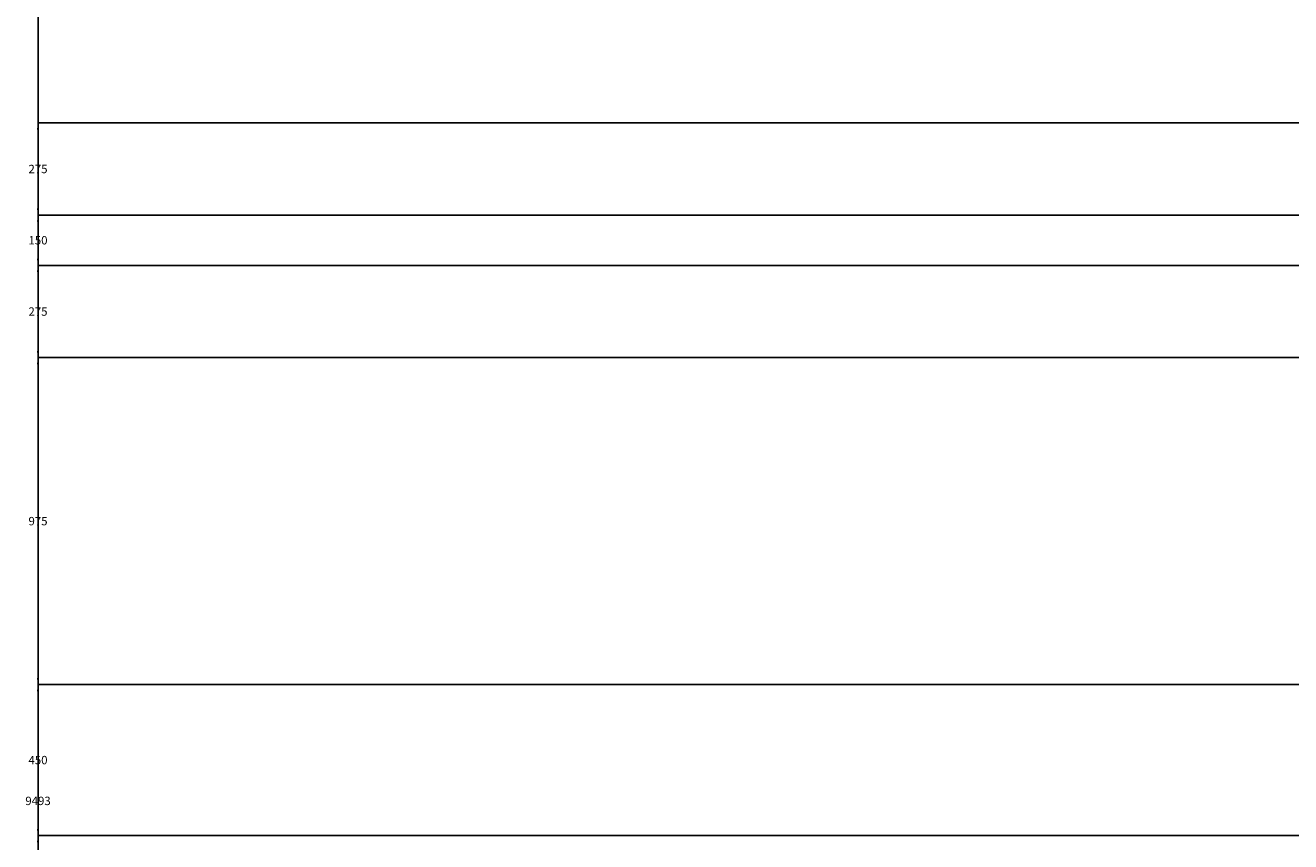
# Model space of a CAD drawing. Units: millimetres. Extents: x -692 to 9639, y -141 to 10345.
# Tile 11 of 19: x -687 to 3088, y 4981 to 7415. Entities that reach past the tile are written whole.
import ezdxf

# ---------------------------------------------------------------- set-up
doc = ezdxf.new("R2010")
doc.units = ezdxf.units.MM
doc.header["$MEASUREMENT"] = 0
doc.layers.add('A-ANNO-DIMS', color=2, linetype='Continuous', lineweight=18)
doc.styles.get("Standard").update_dxf_attribs({"font": 'arial.ttf'})
doc.dimstyles.get("Standard").update_dxf_attribs({"dimtxt": 25, "dimasz": 20, "dimexe": 0.18, "dimexo": 10, "dimgap": 10, "dimtad": 0, "dimtih": 1, "dimtoh": 1, "dimdec": 0, "dimzin": 0, "dimdsep": 46, "dimtxsty": 'Standard', "dimcen": 10, "dimadec": 0, "dimazin": 0, "dimtfac": 1, "dimtdec": 0, "dimtofl": 0, "dimtmove": 0, "dimatfit": 3, "dimfxl": 1, "dimtolj": 1, "dimtzin": 0, "dimarcsym": 0})

# ---------------------------------------------------------------- blocks, each defined once
blk = doc.blocks.new('*D7')
at = {"layer": 'A-ANNO-DIMS', "color": 0, "lineweight": -2, "transparency": 16777216}
for p, q in [((8481.5, 9848.8), (-649.1, 9848.8)), ((-648.9, 9828.8), (-648.9, 5124.9)), ((-648.9, 375.6), (-648.9, 5079.4)), ((2463.7, 355.6), (-649.1, 355.6))]:
    blk.add_line(p, q, dxfattribs=at)
at = {"layer": 'A-ANNO-DIMS', "color": 0, "lineweight": -3, "transparency": 16777216}
for points in [[(-652.2, 9828.8), (-645.6, 9828.8), (-648.9, 9848.8)], [(-652.2, 375.6), (-645.6, 375.6), (-648.9, 355.6)]]:
    blk.add_solid(points, dxfattribs=at)
at = {"layer": 'Defpoints', "color": 0, "lineweight": -3, "transparency": 16777216}
for p in [(-648.9, 9848.8), (8491.5, 9848.8), (2473.7, 355.6)]:
    blk.add_point(p, dxfattribs=at)
at = {"layer": 'A-ANNO-DIMS', "color": 0, "transparency": 16777216, "insert": (-648.9, 5102.2), "char_height": 25, "attachment_point": 5}
blk.add_mtext('\\A1;9493', dxfattribs=at)
blk = doc.blocks.new('*D63')
at = {"layer": 'A-ANNO-DIMS', "color": 0, "lineweight": -2, "transparency": 16777216}
for p, q in [((3931.5, 4998.8), (-649.1, 4998.8)), ((-648.9, 4978.8), (-648.9, 4946.5)), ((-648.9, 4868.8), (-648.9, 4901)), ((3781.5, 4848.8), (-649.1, 4848.8))]:
    blk.add_line(p, q, dxfattribs=at)
at = {"layer": 'A-ANNO-DIMS', "color": 0, "lineweight": -3, "transparency": 16777216}
for points in [[(-652.2, 4978.8), (-645.6, 4978.8), (-648.9, 4998.8)], [(-652.2, 4868.8), (-645.6, 4868.8), (-648.9, 4848.8)]]:
    blk.add_solid(points, dxfattribs=at)
at = {"layer": 'Defpoints', "color": 0, "lineweight": -3, "transparency": 16777216}
for p in [(-648.9, 4998.8), (3941.5, 4998.8), (3791.5, 4848.8)]:
    blk.add_point(p, dxfattribs=at)
at = {"layer": 'A-ANNO-DIMS', "color": 0, "transparency": 16777216, "insert": (-648.9, 4923.8), "char_height": 25, "attachment_point": 5}
blk.add_mtext('\\A1;150', dxfattribs=at)
blk = doc.blocks.new('*D64')
at = {"layer": 'A-ANNO-DIMS', "color": 0, "lineweight": -2, "transparency": 16777216}
for p, q in [((3996.3, 5448.8), (-649.1, 5448.8)), ((-648.9, 5428.8), (-648.9, 5246.5)), ((-648.9, 5018.8), (-648.9, 5201)), ((3931.5, 4998.8), (-649.1, 4998.8))]:
    blk.add_line(p, q, dxfattribs=at)
at = {"layer": 'A-ANNO-DIMS', "color": 0, "lineweight": -3, "transparency": 16777216}
for points in [[(-652.2, 5428.8), (-645.6, 5428.8), (-648.9, 5448.8)], [(-652.2, 5018.8), (-645.6, 5018.8), (-648.9, 4998.8)]]:
    blk.add_solid(points, dxfattribs=at)
at = {"layer": 'Defpoints', "color": 0, "lineweight": -3, "transparency": 16777216}
for p in [(-648.9, 5448.8), (4006.3, 5448.8), (3941.5, 4998.8)]:
    blk.add_point(p, dxfattribs=at)
at = {"layer": 'A-ANNO-DIMS', "color": 0, "transparency": 16777216, "insert": (-648.9, 5223.8), "char_height": 25, "attachment_point": 5}
blk.add_mtext('\\A1;450', dxfattribs=at)
blk = doc.blocks.new('*D65')
at = {"layer": 'A-ANNO-DIMS', "color": 0, "lineweight": -2, "transparency": 16777216}
for p, q in [((3996.3, 6423.8), (-649.1, 6423.8)), ((-648.9, 6403.8), (-648.9, 5959)), ((-648.9, 5468.8), (-648.9, 5913.5)), ((3996.3, 5448.8), (-649.1, 5448.8))]:
    blk.add_line(p, q, dxfattribs=at)
at = {"layer": 'A-ANNO-DIMS', "color": 0, "lineweight": -3, "transparency": 16777216}
for points in [[(-652.2, 6403.8), (-645.6, 6403.8), (-648.9, 6423.8)], [(-652.2, 5468.8), (-645.6, 5468.8), (-648.9, 5448.8)]]:
    blk.add_solid(points, dxfattribs=at)
at = {"layer": 'Defpoints', "color": 0, "lineweight": -3, "transparency": 16777216}
for p in [(-648.9, 6423.8), (4006.3, 6423.8), (4006.3, 5448.8)]:
    blk.add_point(p, dxfattribs=at)
at = {"layer": 'A-ANNO-DIMS', "color": 0, "transparency": 16777216, "insert": (-648.9, 5936.3), "char_height": 25, "attachment_point": 5}
blk.add_mtext('\\A1;975', dxfattribs=at)
blk = doc.blocks.new('*D66')
at = {"layer": 'A-ANNO-DIMS', "color": 0, "lineweight": -2, "transparency": 16777216}
for p, q in [((3931.5, 6698.8), (-649.1, 6698.8)), ((-648.9, 6678.8), (-648.9, 6584)), ((-648.9, 6443.8), (-648.9, 6538.5)), ((3996.3, 6423.8), (-649.1, 6423.8))]:
    blk.add_line(p, q, dxfattribs=at)
at = {"layer": 'A-ANNO-DIMS', "color": 0, "lineweight": -3, "transparency": 16777216}
for points in [[(-652.2, 6678.8), (-645.6, 6678.8), (-648.9, 6698.8)], [(-652.2, 6443.8), (-645.6, 6443.8), (-648.9, 6423.8)]]:
    blk.add_solid(points, dxfattribs=at)
at = {"layer": 'Defpoints', "color": 0, "lineweight": -3, "transparency": 16777216}
for p in [(-648.9, 6698.8), (3941.5, 6698.8), (4006.3, 6423.8)]:
    blk.add_point(p, dxfattribs=at)
at = {"layer": 'A-ANNO-DIMS', "color": 0, "transparency": 16777216, "insert": (-648.9, 6561.3), "char_height": 25, "attachment_point": 5}
blk.add_mtext('\\A1;275', dxfattribs=at)
blk = doc.blocks.new('*D67')
at = {"layer": 'A-ANNO-DIMS', "color": 0, "lineweight": -2, "transparency": 16777216}
for p, q in [((3781.5, 6848.8), (-649.1, 6848.8)), ((-648.9, 6828.8), (-648.9, 6796.5)), ((-648.9, 6718.8), (-648.9, 6751)), ((3931.5, 6698.8), (-649.1, 6698.8))]:
    blk.add_line(p, q, dxfattribs=at)
at = {"layer": 'A-ANNO-DIMS', "color": 0, "lineweight": -3, "transparency": 16777216}
for points in [[(-652.2, 6828.8), (-645.6, 6828.8), (-648.9, 6848.8)], [(-652.2, 6718.8), (-645.6, 6718.8), (-648.9, 6698.8)]]:
    blk.add_solid(points, dxfattribs=at)
at = {"layer": 'Defpoints', "color": 0, "lineweight": -3, "transparency": 16777216}
for p in [(-648.9, 6848.8), (3791.5, 6848.8), (3941.5, 6698.8)]:
    blk.add_point(p, dxfattribs=at)
at = {"layer": 'A-ANNO-DIMS', "color": 0, "transparency": 16777216, "insert": (-648.9, 6773.8), "char_height": 25, "attachment_point": 5}
blk.add_mtext('\\A1;150', dxfattribs=at)
blk = doc.blocks.new('*D68')
at = {"layer": 'A-ANNO-DIMS', "color": 0, "lineweight": -2, "transparency": 16777216}
for p, q in [((3931.5, 7123.8), (-649.1, 7123.8)), ((-648.9, 7103.8), (-648.9, 7009)), ((-648.9, 6868.8), (-648.9, 6963.5)), ((3781.5, 6848.8), (-649.1, 6848.8))]:
    blk.add_line(p, q, dxfattribs=at)
at = {"layer": 'A-ANNO-DIMS', "color": 0, "lineweight": -3, "transparency": 16777216}
for points in [[(-652.2, 7103.8), (-645.6, 7103.8), (-648.9, 7123.8)], [(-652.2, 6868.8), (-645.6, 6868.8), (-648.9, 6848.8)]]:
    blk.add_solid(points, dxfattribs=at)
at = {"layer": 'Defpoints', "color": 0, "lineweight": -3, "transparency": 16777216}
for p in [(-648.9, 7123.8), (3941.5, 7123.8), (3791.5, 6848.8)]:
    blk.add_point(p, dxfattribs=at)
at = {"layer": 'A-ANNO-DIMS', "color": 0, "transparency": 16777216, "insert": (-648.9, 6986.3), "char_height": 25, "attachment_point": 5}
blk.add_mtext('\\A1;275', dxfattribs=at)

msp = doc.modelspace()

# ---------------------------------------------------------------- dimensions: what is measured, and where the dimension line sits
at = {"layer": 'A-ANNO-DIMS'}
for base, p1, p2, picture, middle in [((-648.912, 9848.772), (2473.746, 355.575), (8491.547, 9848.772), '*D7', (-648.912, 5102.173)), ((-648.912, 7123.772), (3791.547, 6848.772), (3941.547, 7123.772), '*D68', (-648.912, 6986.272)), ((-648.912, 6848.772), (3941.547, 6698.772), (3791.547, 6848.772), '*D67', (-648.912, 6773.772)), ((-648.912, 6698.772), (4006.259, 6423.772), (3941.547, 6698.772), '*D66', (-648.912, 6561.272)), ((-648.912, 6423.772), (4006.259, 5448.772), (4006.259, 6423.772), '*D65', (-648.912, 5936.272)), ((-648.912, 5448.772), (3941.547, 4998.772), (4006.259, 5448.772), '*D64', (-648.912, 5223.772)), ((-648.912, 4998.772), (3791.547, 4848.772), (3941.547, 4998.772), '*D63', (-648.912, 4923.772))]:
    dim = msp.add_linear_dim(base=base, p1=p1, p2=p2, angle=90, dimstyle='Standard', override={"dimdec": 0, "dimlfac": 1, "dimrnd": 0, "dimzin": 0, "dimdsep": 46, "dimlunit": 2}, dxfattribs=at)
    dim.commit()
    dim.dimension.update_dxf_attribs({"geometry": picture, "text_midpoint": middle})

doc.saveas('drawing.dxf')
